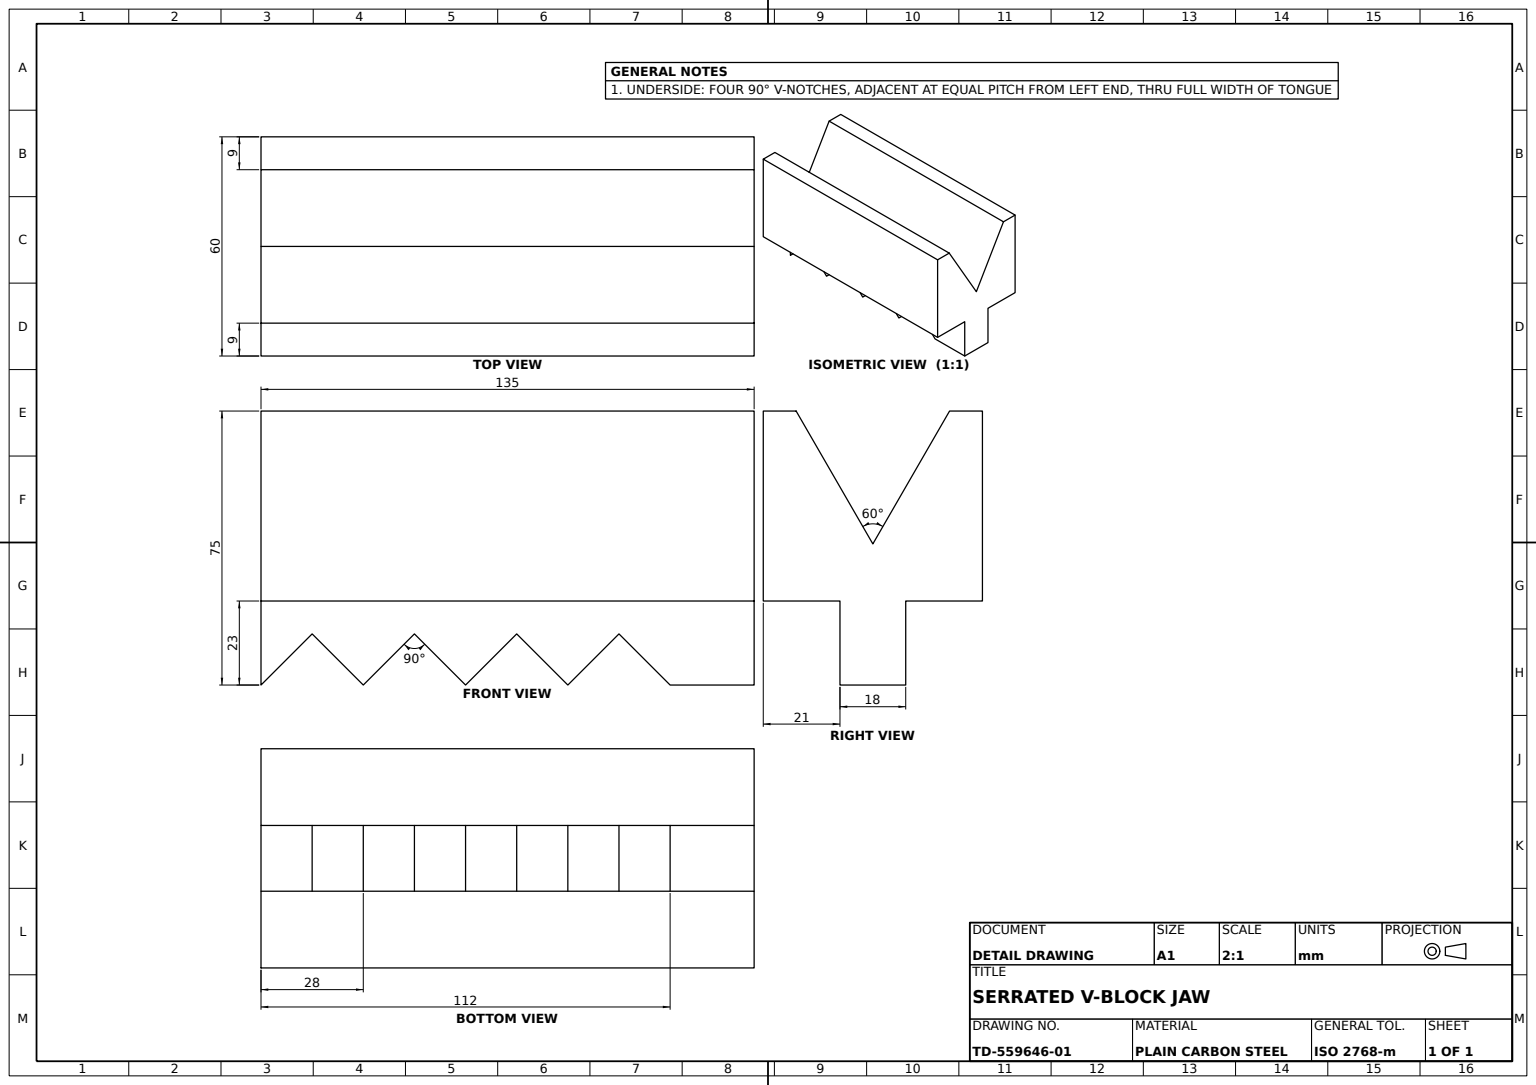
from build123d import *

# Parameters (mm, degrees)
V_BLOCK_BODY_DEPTH          = 135
UNDERSIDE_NOTCHES_CUT_DEPTH = 195


with BuildPart() as part:
    # V-Block Profile Sketch → V-Block Body (new body)
    with BuildSketch(Plane(origin=(0, 0, 0), x_dir=(0, 0, -1), z_dir=(1, 0, 0))):
        Polygon((-30, 52), (-30, 0), (-9, 0), (-9, -23), (9, -23), (9, 0), (30, 0), (30, 52), (21, 52), (0, 15.626933041), (-21, 52), align=None)
    extrude(amount=-V_BLOCK_BODY_DEPTH)

    # Underside Notches Sketch → Underside Notches Cut (cut)
    with BuildSketch(Plane.XY.offset(9)):
        Polygon((-135, -23), (-121, -9), (-107, -23), (-93, -9), (-79, -23), (-65, -9), (-51, -23), (-37, -9), (-7.657800388, -38.342199612), (-135, -44.429564146), align=None)
    extrude(amount=-UNDERSIDE_NOTCHES_CUT_DEPTH, mode=Mode.SUBTRACT)


solid = part.part
